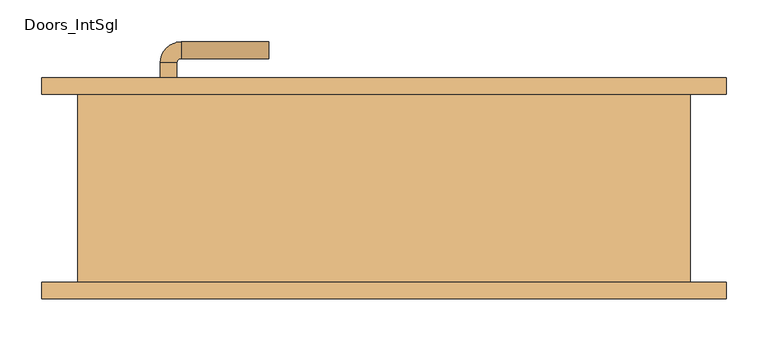
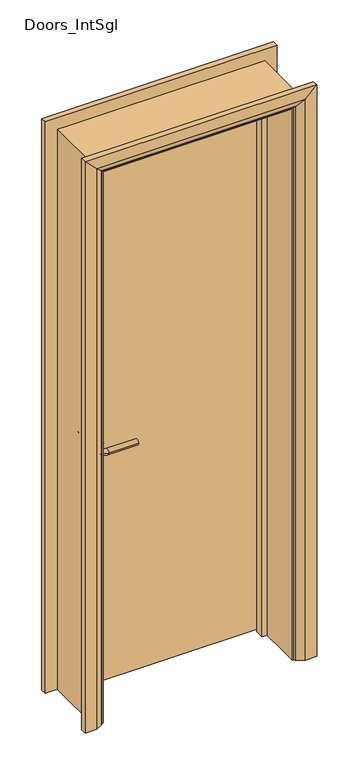
"""IFC4 building model written with IfcOpenShell, lengths in millimetres: door geometry, Doors_IntSgl."""

from ifc_helpers import new_model, si_unit, point, frame, frame_2d, origin, place, context, project, spatial, polyline, circle_curve, ellipse_curve, trimmed, segment, composite_curve, outline, extrude, faceted_brep, source, transform, mapped, element, save
from ifc_brep_helpers import plane_surface, cylinder_surface, revolved_surface, advanced_brep


def doors_intsgl_1caea894(model_context):
    return source(origin(), model_context, "Body", "SolidModel", [
        advanced_brep(
        [(-268.0, 66.5, 900.0), (-248.0, 66.5, 900.0), (-248.0, 36.5, 900.0), (-268.0, 36.5, 900.0), (-243.0, 31.5, 900.0), (-243.0, 11.5, 900.0), (-138.0, 11.5, 900.0), (-138.0, 31.5, 900.0)],
        [
            (0, 1, circle_curve(frame((-258.0, 66.5, 900.0), z_axis=(0.0, 1.0, 0.0), x_axis=(1.0, 0.0, 0.0)), 10.0)),
            (1, 0, circle_curve(frame((-258.0, 66.5, 900.0), z_axis=(0.0, 1.0, 0.0), x_axis=(1.0, 0.0, 0.0)), 10.0)),
            (1, 2),
            (2, 3, circle_curve(frame((-258.0, 36.5, 900.0), z_axis=(0.0, 1.0, 0.0), x_axis=(1.0, 0.0, 0.0)), 10.0)),
            (3, 0),
            (3, 2, circle_curve(frame((-258.0, 36.5, 900.0), z_axis=(0.0, 1.0, 0.0), x_axis=(1.0, 0.0, 0.0)), 10.0)),
            (4, 5, circle_curve(frame((-243.0, 21.5, 900.0), z_axis=(-1.0, 0.0, 0.0), x_axis=(0.0, 1.0, 0.0)), 10.0)),
            (5, 3, circle_curve(frame((-243.0, 36.5, 900.0), z_axis=(0.0, 0.0, -1.0), x_axis=(-1.0, 0.0, 0.0)), 25.0)),
            (2, 4, circle_curve(frame((-243.0, 36.5, 900.0), z_axis=(0.0, 0.0, 1.0), x_axis=(-1.0, 0.0, 0.0)), 5.0)),
            (5, 4, circle_curve(frame((-243.0, 21.5, 900.0), z_axis=(-1.0, 0.0, 0.0), x_axis=(0.0, 1.0, 0.0)), 10.0)),
            (6, 7, circle_curve(frame((-138.0, 21.5, 900.0), z_axis=(1.0, 0.0, 0.0), x_axis=(0.0, 1.0, 0.0)), 10.0)),
            (7, 6, circle_curve(frame((-138.0, 21.5, 900.0), z_axis=(1.0, 0.0, 0.0), x_axis=(0.0, 1.0, 0.0)), 10.0)),
            (4, 7),
            (6, 5),
        ],
        [
            plane_surface(frame((-258.0, 66.5, 900.0), z_axis=(0.0, 1.0, 0.0), x_axis=(0.0, 0.0, 1.0))),
            cylinder_surface(frame((-258.0, 66.5, 900.0), z_axis=(0.0, 1.0, 0.0), x_axis=(1.0, 0.0, 0.0)), 10.0),
            revolved_surface(trimmed(ellipse_curve(frame((-258.0, 36.5, 900.0), z_axis=(0.0, -1.0, 0.0), x_axis=(1.0, 0.0, 0.0)), 10.0, 10.0), [point((-268.0, 36.5, 900.0))], [point((-248.0, 36.5, 900.0))], True, "CARTESIAN"), (-243.0, 36.5, 900.0), (0.0, 0.0, -1.0)),
            revolved_surface(trimmed(ellipse_curve(frame((-258.0, 36.5, 900.0), z_axis=(0.0, -1.0, 0.0), x_axis=(1.0, 0.0, 0.0)), 10.0, 10.0), [point((-248.0, 36.5, 900.0))], [point((-268.0, 36.5, 900.0))], True, "CARTESIAN"), (-243.0, 36.5, 900.0), (0.0, 0.0, -1.0)),
            plane_surface(frame((-138.0, 21.5, 900.0), z_axis=(1.0, 0.0, 0.0), x_axis=(0.0, 0.0, 1.0))),
            cylinder_surface(frame((-243.0, 21.5, 900.0), z_axis=(-1.0, 0.0, 0.0), x_axis=(0.0, 1.0, 0.0)), 10.0),
        ],
        [
            (0, [[1, 2]]),
            (1, [[3, 4, 5, -2]]),
            (1, [[-5, 6, -3, -1]]),
            (2, [[7, 8, -4, 9]]),
            (3, [[10, -9, -6, -8]]),
            (4, [[11, 12]]),
            (5, [[13, -11, 14, -7]]),
            (5, [[-14, -12, -13, -10]]),
        ],
    ),
        extrude(outline(composite_curve([segment(trimmed(circle_curve(frame_2d((900.0, -260.5)), 30.0), [point((900.0, -290.5))], [point((900.0, -230.5))], False, "CARTESIAN"), True, "CONTINUOUS"), segment(trimmed(circle_curve(frame_2d((900.0, -260.5)), 30.0), [point((900.0, -230.5))], [point((900.0, -290.5))], False, "CARTESIAN"), True, "CONTINUOUS")], self_intersect=False)), frame((0.0, 66.5, 0.0), z_axis=(0.0, 1.0, 0.0), x_axis=(0.0, 0.0, 1.0)), (0.0, 0.0, 1.0), 8.0),
        advanced_brep(
        [(-268.0, 120.5, 900.0), (-248.0, 120.5, 900.0), (-268.0, 150.5, 900.0), (-248.0, 150.5, 900.0), (-243.0, 155.5, 900.0), (-243.0, 175.5, 900.0), (-138.0, 175.5, 900.0), (-138.0, 155.5, 900.0)],
        [
            (0, 1, circle_curve(frame((-258.0, 120.5, 900.0), z_axis=(0.0, -1.0, 0.0), x_axis=(1.0, 0.0, 0.0)), 10.0)),
            (1, 0, circle_curve(frame((-258.0, 120.5, 900.0), z_axis=(0.0, -1.0, 0.0), x_axis=(1.0, 0.0, 0.0)), 10.0)),
            (0, 2),
            (2, 3, circle_curve(frame((-258.0, 150.5, 900.0), z_axis=(0.0, -1.0, 0.0), x_axis=(1.0, 0.0, 0.0)), 10.0)),
            (3, 1),
            (3, 2, circle_curve(frame((-258.0, 150.5, 900.0), z_axis=(0.0, -1.0, 0.0), x_axis=(1.0, 0.0, 0.0)), 10.0)),
            (4, 3, circle_curve(frame((-243.0, 150.5, 900.0), z_axis=(0.0, 0.0, 1.0), x_axis=(-1.0, 0.0, 0.0)), 5.0)),
            (2, 5, circle_curve(frame((-243.0, 150.5, 900.0), z_axis=(0.0, 0.0, -1.0), x_axis=(-1.0, 0.0, 0.0)), 25.0)),
            (5, 4, circle_curve(frame((-243.0, 165.5, 900.0), z_axis=(-1.0, 0.0, 0.0), x_axis=(0.0, -1.0, 0.0)), 10.0)),
            (4, 5, circle_curve(frame((-243.0, 165.5, 900.0), z_axis=(-1.0, 0.0, 0.0), x_axis=(0.0, -1.0, 0.0)), 10.0)),
            (6, 7, circle_curve(frame((-138.0, 165.5, 900.0), z_axis=(1.0, 0.0, 0.0), x_axis=(0.0, -1.0, 0.0)), 10.0)),
            (7, 6, circle_curve(frame((-138.0, 165.5, 900.0), z_axis=(1.0, 0.0, 0.0), x_axis=(0.0, -1.0, 0.0)), 10.0)),
            (5, 6),
            (7, 4),
        ],
        [
            plane_surface(frame((-258.0, 120.5, 900.0), z_axis=(0.0, -1.0, 0.0), x_axis=(0.0, 0.0, 1.0))),
            cylinder_surface(frame((-258.0, 120.5, 900.0), z_axis=(0.0, -1.0, 0.0), x_axis=(1.0, 0.0, 0.0)), 10.0),
            revolved_surface(trimmed(ellipse_curve(frame((-258.0, 150.5, 900.0), z_axis=(0.0, -1.0, 0.0), x_axis=(1.0, 0.0, 0.0)), 10.0, 10.0), [point((-268.0, 150.5, 900.0))], [point((-248.0, 150.5, 900.0))], True, "CARTESIAN"), (-243.0, 150.5, 900.0), (0.0, 0.0, -1.0)),
            revolved_surface(trimmed(ellipse_curve(frame((-258.0, 150.5, 900.0), z_axis=(0.0, -1.0, 0.0), x_axis=(1.0, 0.0, 0.0)), 10.0, 10.0), [point((-248.0, 150.5, 900.0))], [point((-268.0, 150.5, 900.0))], True, "CARTESIAN"), (-243.0, 150.5, 900.0), (0.0, 0.0, -1.0)),
            plane_surface(frame((-138.0, 165.5, 900.0), z_axis=(1.0, 0.0, 0.0), x_axis=(0.0, 0.0, 1.0))),
            cylinder_surface(frame((-243.0, 165.5, 900.0), z_axis=(-1.0, 0.0, 0.0), x_axis=(0.0, -1.0, 0.0)), 10.0),
        ],
        [
            (0, [[1, 2]]),
            (1, [[-1, 3, 4, 5]]),
            (1, [[-2, -5, 6, -3]]),
            (2, [[7, -4, 8, 9]]),
            (3, [[-8, -6, -7, 10]]),
            (4, [[11, 12]]),
            (5, [[-9, 13, -12, 14]]),
            (5, [[-10, -14, -11, -13]]),
        ],
    ),
        extrude(outline(composite_curve([segment(trimmed(circle_curve(frame_2d((900.0, -260.5)), 30.0), [point((900.0, -290.5))], [point((900.0, -230.5))], False, "CARTESIAN"), True, "CONTINUOUS"), segment(trimmed(circle_curve(frame_2d((900.0, -260.5)), 30.0), [point((900.0, -230.5))], [point((900.0, -290.5))], False, "CARTESIAN"), True, "CONTINUOUS")], self_intersect=False)), frame((0.0, 112.5, 0.0), z_axis=(0.0, 1.0, 0.0), x_axis=(0.0, 0.0, 1.0)), (0.0, 0.0, 1.0), 8.0),
        extrude(outline(polyline([(333.0, 74.5), (-333.0, 74.5), (-333.0, 112.5), (333.0, 112.5), (333.0, 74.5)])), frame((0.0, 0.0, 8.0), z_axis=(0.0, 0.0, 1.0), x_axis=(1.0, 0.0, 0.0)), (0.0, 0.0, 1.0), 2050.0),
        faceted_brep([(-335.0, 112.5, 0.0), (-335.0, -112.5, 0.0), (-367.0, -112.5, 0.0), (-367.0, 112.5, 0.0), (-335.0, 112.5, 2060.0), (-335.0, -112.5, 2060.0), (-367.0, -112.5, 2092.0), (-367.0, 112.5, 2092.0), (335.0, 112.5, 0.0), (367.0, 112.5, 0.0), (367.0, -112.5, 0.0), (335.0, -112.5, 0.0), (335.0, 112.5, 2060.0), (367.0, 112.5, 2092.0), (367.0, -112.5, 2092.0), (335.0, -112.5, 2060.0)], [[[0, 1, 2, 3]], [[1, 0, 4, 5]], [[2, 1, 5, 6]], [[3, 2, 6, 7]], [[0, 3, 7, 4]], [[8, 9, 10, 11]], [[12, 13, 9, 8]], [[13, 14, 10, 9]], [[14, 15, 11, 10]], [[15, 12, 8, 11]], [[5, 4, 12, 15]], [[6, 5, 15, 14]], [[7, 6, 14, 13]], [[4, 7, 13, 12]]]),
        advanced_brep(
        [(-410.0, -132.5, 0.0), (-410.0, -112.5, 0.0), (-340.0, -112.5, 0.0), (-344.0, -118.5, 0.0), (-370.0, -132.5, 0.0), (-410.0, -132.5, 2135.0), (-410.0, -112.5, 2135.0), (-340.0, -112.5, 2065.0), (-344.0, -118.5, 2069.0), (-370.0, -132.5, 2095.0), (410.0, -132.5, 0.0), (370.0, -132.5, 0.0), (344.0, -118.5, 0.0), (340.0, -112.5, 0.0), (410.0, -112.5, 0.0), (410.0, -132.5, 2135.0), (370.0, -132.5, 2095.0), (344.0, -118.5, 2069.0), (340.0, -112.5, 2065.0), (410.0, -112.5, 2135.0)],
        [
            (0, 1),
            (1, 2),
            (2, 3, circle_curve(frame((-348.0, -111.5, 0.0), z_axis=(0.0, 0.0, -1.0), x_axis=(-1.0, 0.0, 0.0)), 8.0622577)),
            (3, 4),
            (4, 0),
            (0, 5),
            (5, 6),
            (6, 1),
            (6, 7),
            (7, 2),
            (7, 8, ellipse_curve(frame((-348.0, -111.5, 2073.0), z_axis=(-0.7071067811865475, 0.0, -0.7071067811865475), x_axis=(0.7071067811865474, 0.0, -0.7071067811865476)), 11.4017543, 8.0622577)),
            (8, 3),
            (8, 9),
            (9, 4),
            (9, 5),
            (10, 11),
            (11, 12),
            (12, 13, circle_curve(frame((348.0, -111.5, 0.0), z_axis=(0.0, 0.0, -1.0), x_axis=(1.0, 0.0, 0.0)), 8.0622577)),
            (13, 14),
            (14, 10),
            (15, 16),
            (16, 11),
            (10, 15),
            (16, 17),
            (17, 12),
            (17, 18, ellipse_curve(frame((348.0, -111.5, 2073.0), z_axis=(0.7071067811865475, 0.0, -0.7071067811865475), x_axis=(0.7071067811865474, 0.0, 0.7071067811865476)), 11.4017543, 8.0622577)),
            (18, 13),
            (18, 19),
            (19, 14),
            (19, 15),
            (5, 15),
            (19, 6),
            (18, 7),
            (17, 8),
            (16, 9),
        ],
        [
            plane_surface(frame((-340.0, -185.3010989, 0.0), z_axis=(0.0, 0.0, -1.0), x_axis=(1.0, 0.0, 0.0))),
            plane_surface(frame((-410.0, -132.5, 0.0), z_axis=(-1.0, 0.0, 0.0), x_axis=(0.0, 0.0, 1.0))),
            plane_surface(frame((-410.0, -112.5, 0.0), z_axis=(0.0, 1.0, 0.0), x_axis=(0.0, 0.0, 1.0))),
            cylinder_surface(frame((-348.0, -111.5, 0.0), z_axis=(0.0, 0.0, -1.0), x_axis=(-1.0, 0.0, 0.0)), 8.0622577),
            plane_surface(frame((-344.0, -118.5, 0.0), z_axis=(0.4740998230350183, -0.8804710999221749, 0.0), x_axis=(0.0, 0.0, 1.0))),
            plane_surface(frame((-370.0, -132.5, 0.0), z_axis=(0.0, -1.0, 0.0), x_axis=(0.0, 0.0, 1.0))),
            plane_surface(frame((340.0, -185.3010989, 0.0), z_axis=(0.0, 0.0, -1.0), x_axis=(-1.0, 0.0, 0.0))),
            plane_surface(frame((370.0, -132.5, 2095.0), z_axis=(0.0, -1.0, 0.0), x_axis=(0.0, 0.0, -1.0))),
            plane_surface(frame((344.0, -118.5, 2069.0), z_axis=(-0.4740998230350183, -0.8804710999221749, 0.0), x_axis=(0.0, 0.0, -1.0))),
            cylinder_surface(frame((348.0, -111.5, 2065.0), z_axis=(0.0, 0.0, 1.0), x_axis=(1.0, 0.0, 0.0)), 8.0622577),
            plane_surface(frame((410.0, -112.5, 2135.0), z_axis=(0.0, 1.0, 0.0), x_axis=(0.0, 0.0, -1.0))),
            plane_surface(frame((410.0, -132.5, 2135.0), z_axis=(1.0, 0.0, 0.0), x_axis=(0.0, 0.0, -1.0))),
            plane_surface(frame((-410.0, -132.5, 2135.0), z_axis=(0.0, 0.0, 1.0), x_axis=(1.0, 0.0, 0.0))),
            plane_surface(frame((-410.0, -112.5, 2135.0), z_axis=(0.0, 1.0, 0.0), x_axis=(1.0, 0.0, 0.0))),
            cylinder_surface(frame((-340.0, -111.5, 2073.0), z_axis=(-1.0, 0.0, 0.0), x_axis=(0.0, 0.0, 1.0)), 8.0622577),
            plane_surface(frame((-344.0, -118.5, 2069.0), z_axis=(0.0, -0.8804710999221749, -0.4740998230350183), x_axis=(1.0, 0.0, 0.0))),
            plane_surface(frame((-370.0, -132.5, 2095.0), z_axis=(0.0, -1.0, 0.0), x_axis=(1.0, 0.0, 0.0))),
        ],
        [
            (0, [[1, 2, 3, 4, 5]]),
            (1, [[-1, 6, 7, 8]]),
            (2, [[-2, -8, 9, 10]]),
            (3, [[-3, -10, 11, 12]]),
            (4, [[-4, -12, 13, 14]]),
            (5, [[-5, -14, 15, -6]]),
            (6, [[16, 17, 18, 19, 20]]),
            (7, [[21, 22, -16, 23]]),
            (8, [[24, 25, -17, -22]]),
            (9, [[26, 27, -18, -25]]),
            (10, [[28, 29, -19, -27]]),
            (11, [[30, -23, -20, -29]]),
            (12, [[-7, 31, -30, 32]]),
            (13, [[-9, -32, -28, 33]]),
            (14, [[-11, -33, -26, 34]]),
            (15, [[-13, -34, -24, 35]]),
            (16, [[-15, -35, -21, -31]]),
        ],
    ),
        extrude(outline(polyline([(0.0, -335.0), (0.0, -316.0), (2041.0, -316.0), (2041.0, 316.0), (0.0, 316.0), (0.0, 335.0), (2060.0, 335.0), (2060.0, -335.0), (0.0, -335.0)])), frame((0.0, 40.5, 0.0), z_axis=(0.0, 1.0, 0.0), x_axis=(0.0, 0.0, 1.0)), (0.0, 0.0, 1.0), 32.0),
        advanced_brep(
        [(410.0, 132.5, 0.0), (410.0, 112.5, 0.0), (340.0, 112.5, 0.0), (344.0, 118.5, 0.0), (370.0, 132.5, 0.0), (410.0, 132.5, 2135.0), (410.0, 112.5, 2135.0), (-410.0, 112.5, 2135.0), (-410.0, 112.5, 0.0), (-340.0, 112.5, 0.0), (-340.0, 112.5, 2065.0), (340.0, 112.5, 2065.0), (344.0, 118.5, 2069.0), (370.0, 132.5, 2095.0), (-370.0, 132.5, 2095.0), (-370.0, 132.5, 0.0), (-410.0, 132.5, 0.0), (-410.0, 132.5, 2135.0), (-344.0, 118.5, 0.0), (-344.0, 118.5, 2069.0)],
        [
            (0, 1),
            (1, 2),
            (2, 3, circle_curve(frame((348.0, 111.5, 0.0), z_axis=(0.0, 0.0, -1.0), x_axis=(1.0, 0.0, 0.0)), 8.0622577)),
            (3, 4),
            (4, 0),
            (0, 5),
            (5, 6),
            (6, 1),
            (6, 7),
            (7, 8),
            (8, 9),
            (9, 10),
            (10, 11),
            (11, 2),
            (11, 12, ellipse_curve(frame((348.0, 111.5, 2073.0), z_axis=(0.7071067811865475, 0.0, -0.7071067811865475), x_axis=(-0.7071067811865474, 0.0, -0.7071067811865476)), 11.4017543, 8.0622577)),
            (12, 3),
            (12, 13),
            (13, 4),
            (13, 14),
            (14, 15),
            (15, 16),
            (16, 17),
            (17, 5),
            (7, 17),
            (16, 8),
            (15, 18),
            (18, 9, circle_curve(frame((-348.0, 111.5, 0.0), z_axis=(0.0, 0.0, -1.0), x_axis=(-1.0, 0.0, 0.0)), 8.0622577)),
            (19, 10, ellipse_curve(frame((-348.0, 111.5, 2073.0), z_axis=(-0.7071067811865475, 0.0, -0.7071067811865475), x_axis=(-0.7071067811865474, 0.0, 0.7071067811865476)), 11.4017543, 8.0622577)),
            (18, 19),
            (14, 19),
            (19, 12),
        ],
        [
            plane_surface(frame((340.0, 112.5, 0.0), z_axis=(0.0, 0.0, -1.0), x_axis=(0.0, -1.0, 0.0))),
            plane_surface(frame((410.0, 132.5, 0.0), z_axis=(1.0, 0.0, 0.0), x_axis=(0.0, 0.0, 1.0))),
            plane_surface(frame((410.0, 112.5, 0.0), z_axis=(0.0, -1.0, 0.0), x_axis=(0.0, 0.0, 1.0))),
            cylinder_surface(frame((348.0, 111.5, 0.0), z_axis=(0.0, 0.0, -1.0), x_axis=(1.0, 0.0, 0.0)), 8.0622577),
            plane_surface(frame((344.0, 118.5, 0.0), z_axis=(-0.4740998230350126, 0.880471099922178, 0.0), x_axis=(0.0, 0.0, 1.0))),
            plane_surface(frame((370.0, 132.5, 0.0), z_axis=(0.0, 1.0, 0.0), x_axis=(0.0, 0.0, 1.0))),
            plane_surface(frame((-410.0, 132.5, 2135.0), z_axis=(-1.0, 0.0, 0.0), x_axis=(0.0, 0.0, -1.0))),
            plane_surface(frame((-340.0, 112.5, 0.0), z_axis=(0.0, 0.0, -1.0), x_axis=(0.0, -1.0, 0.0))),
            cylinder_surface(frame((-348.0, 111.5, 2065.0), z_axis=(0.0, 0.0, 1.0), x_axis=(-1.0, 0.0, 0.0)), 8.0622577),
            plane_surface(frame((-344.0, 118.5, 2069.0), z_axis=(0.47409982303501824, 0.8804710999221749, 0.0), x_axis=(0.0, 0.0, -1.0))),
            plane_surface(frame((410.0, 132.5, 2135.0), z_axis=(0.0, 0.0, 1.0), x_axis=(-1.0, 0.0, 0.0))),
            cylinder_surface(frame((340.0, 111.5, 2073.0), z_axis=(1.0, 0.0, 0.0), x_axis=(0.0, 0.0, 1.0)), 8.0622577),
            plane_surface(frame((344.0, 118.5, 2069.0), z_axis=(0.0, 0.8804710999221764, -0.4740998230350154), x_axis=(-1.0, 0.0, 0.0))),
        ],
        [
            (0, [[1, 2, 3, 4, 5]]),
            (1, [[-1, 6, 7, 8]]),
            (2, [[-2, -8, 9, 10, 11, 12, 13, 14]]),
            (3, [[-3, -14, 15, 16]]),
            (4, [[-4, -16, 17, 18]]),
            (5, [[-5, -18, 19, 20, 21, 22, 23, -6]]),
            (6, [[24, -22, 25, -10]]),
            (7, [[-21, 26, 27, -11, -25]]),
            (8, [[28, -12, -27, 29]]),
            (9, [[30, -29, -26, -20]]),
            (10, [[-7, -23, -24, -9]]),
            (11, [[-15, -13, -28, 31]]),
            (12, [[-17, -31, -30, -19]]),
        ],
    ),
    ])


if __name__ == "__main__":
    model = new_model("IFC4")
    model_context = context("Model", 3, world=origin())
    ifc_project = project(units=[si_unit("LENGTHUNIT", "METRE", prefix="MILLI")], contexts=[model_context])
    site = spatial("IfcSite", under=ifc_project)
    building = spatial("IfcBuilding", under=site)
    placement = place(None, origin())
    doors_intsgl_shape = doors_intsgl_1caea894(model_context)
    element("IfcDoor", 1, ObjectType="Doors_IntSgl", at=placement, inside=building, context=model_context, shape_type="MappedRepresentation", body=[
        mapped(doors_intsgl_shape, transform((0.0, 0.0, 0.0), x_axis=(1.0, 0.0, 0.0), y_axis=(0.0, 1.0, 0.0), z_axis=(0.0, 0.0, 1.0))),
    ])
    save(model, "model.ifc")

# Revit data of these elements
# Type "Doors_IntSgl"
#   Type Mark = "45"
#   Type Comments = "Internal Single"
#   Operation = "SingleSwingRight"
#   Manufacturer = "Revit"
#   Keynote = "L20"
#   Description = "Internal Single Door"
#   Analytic Construction = "Metal"
#   UnderCut = 8 mm
#   Tolerance = 2 mm
#   Thickness = 38 mm
#   Thermal Resistance (R) = 0.270117 (m²·K)/W
#   Structural Tolerance = 8 mm
#   StopDepth = 32 mm
#   Stop Thickness = 19 mm
#   Rough Width = 750 mm
#   Rough Height = 2100 mm
#   Height to Top Lock Rail = 1000 mm
#   Heat Transfer Coefficient (U) = 3.7021 W/(m²·K)
#   Handle Z Distance = 900 mm
#   Handle X Distance = 75 mm
#   Frame Thickness = 32 mm
#   Door Panel Width = 666 mm
#   Door Panel Thickness = 38 mm
#   Door Panel Offset = 0 mm
#   Height = 2100 mm
#   Width = 750 mm
#   Door Panel Height = 2050 mm
#   Architrave Setback = 5 mm
#   Vis - Ironmongery = yes
#   Define Thermal Properties by = 1
#   Material Ironmongery = Door - Handle
#   Material Frame = Door - Frame/Mullion (1)
#   Material Door = Door - Panel
#   Material Architrave = Door - Architrave
#   Visual Light Transmittance = 0
#   Solar Heat Gain Coefficient = 0
#   Function = (empty or 0)
#   Wall Closure = (empty or 0)
# Element 1 (IfcDoor, "Doors_IntSgl")
#   Materials on its faces: "Door - Architrave", "Door - Handle", "Door - Frame/Mullion (1)", "Door - Panel"
# Materials
#   "Door - Handle": colour RGB 0 0 0, transparency 0, Cost = 0
#   "Door - Frame/Mullion (1)": class "Wood", colour RGB 212 179 113, transparency 0, Keynote = "L20", Cost = 0
#   "Door - Panel": class "Wood", colour RGB 210 159 95, transparency 0, Cost = 0
#   "Door - Architrave": class "Wood", colour RGB 154 90 5, transparency 0, Keynote = "P20", Cost = 0
